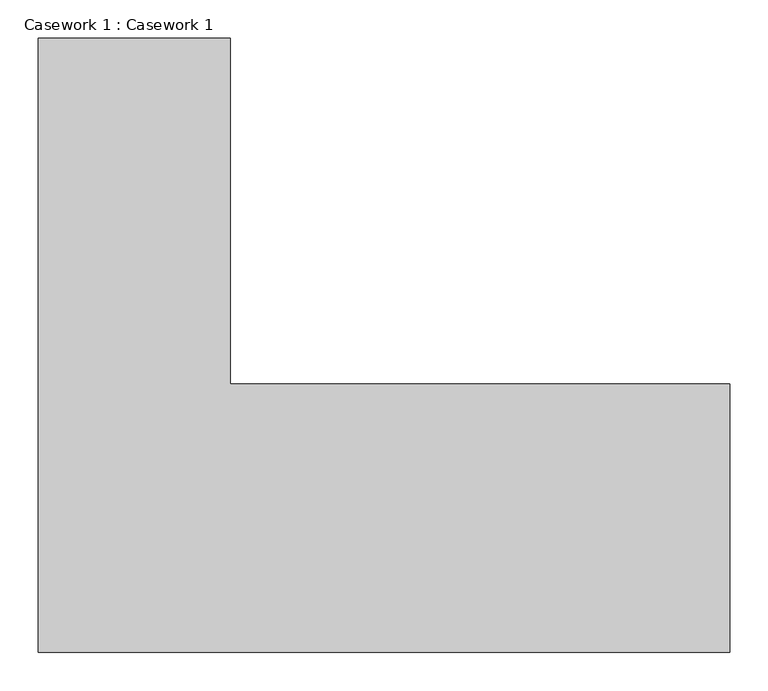
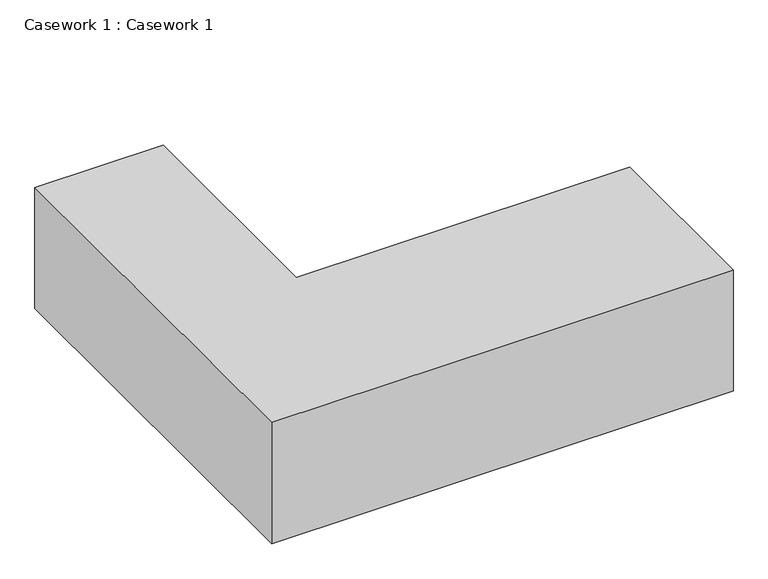
"""IFC4 building model written with IfcOpenShell, lengths in millimetres: furniture geometry, Casework 1 : Casework 1."""

from ifc_helpers import new_model, si_unit, origin, origin_with_axes, place, context, project, spatial, polyline, outline, extrude, source, transform, mapped, element, save


def casework_1_casework_1_f5bf10af(model_context):
    return source(origin(), model_context, "Body", "SweptSolid", [
        extrude(outline(polyline([(7626.1730929, -5475.2269163), (7876.1730929, -5475.2269163), (7876.1730929, -5925.7891179), (8526.1730929, -5925.7891179), (8526.1730929, -6275.2269163), (7626.1730929, -6275.2269163), (7626.1730929, -5475.2269163)])), origin_with_axes(), (0.0, 0.0, 1.0), 250.0),
    ])


if __name__ == "__main__":
    model = new_model("IFC4")
    model_context = context("Model", 3, world=origin())
    ifc_project = project(units=[si_unit("LENGTHUNIT", "METRE", prefix="MILLI")], contexts=[model_context])
    site = spatial("IfcSite", under=ifc_project)
    building = spatial("IfcBuilding", under=site)
    placement = place(None, origin())
    casework_1_casework_1_shape = casework_1_casework_1_f5bf10af(model_context)
    element("IfcFurniture", 1, ObjectType="Casework 1 : Casework 1", at=placement, inside=building, context=model_context, shape_type="MappedRepresentation", body=[
        mapped(casework_1_casework_1_shape, transform((0.0, 0.0, 0.0), x_axis=(1.0, 0.0, 0.0), y_axis=(0.0, 1.0, 0.0), z_axis=(0.0, 0.0, 1.0))),
    ])
    save(model, "model.ifc")
